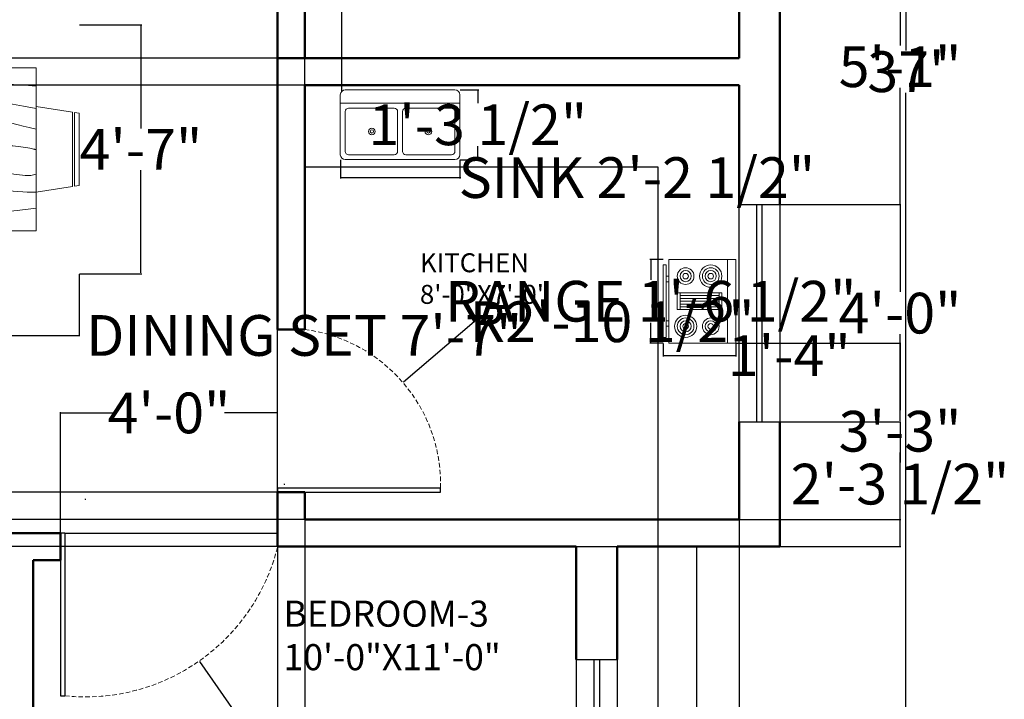
# Model space of a CAD drawing. Units: inches. Extents: x 4033 to 4435, y 499 to 1031.
# Tile 3 of 4: x 4217 to 4435, y 614 to 765. Entities that reach past the tile are written whole.
import ezdxf

# ---------------------------------------------------------------- set-up
doc = ezdxf.new("R2010")
doc.units = ezdxf.units.IN
doc.header["$MEASUREMENT"] = 0
doc.linetypes.add('DASHEDX2', pattern=[1.5, 1, -0.5])
for name, color, linetype, lineweight in [('A-ANNO-DIMS', 2, 'Continuous', 18), ('A-AREA-IDEN', 7, 'Continuous', 18), ('A-DOOR', 3, 'Continuous', 25), ('A-DOOR-SWNG', 3, 'DASHEDX2', 13), ('A-EQPM', 9, 'Continuous', 18), ('A-FLOR-CASE', 8, 'Continuous', 25), ('A-FLOR-FIXT', 8, 'Continuous', 18), ('A-FURN', 8, 'Continuous', 18), ('A-WALL', 7, 'Continuous', 50)]:
    doc.layers.add(name, color=color, linetype=linetype, lineweight=lineweight)
doc.layers.add('A-GLAZ', color=177, linetype='Continuous', lineweight=25, true_color=0x293189)
doc.styles.get("Standard").update_dxf_attribs({"font": 'arial.ttf'})
doc.dimstyles.get("Standard").update_dxf_attribs({"dimtxt": 9, "dimasz": 0.18, "dimexe": 0.18, "dimexo": 0.0625, "dimgap": 0.09, "dimtad": 0, "dimtih": 1, "dimtoh": 1, "dimdec": 0, "dimzin": 0, "dimdsep": 46, "dimlunit": 3, "dimtxsty": 'Standard', "dimcen": 0.09, "dimadec": 0, "dimazin": 0, "dimtfac": 1, "dimtdec": 0, "dimtofl": 0, "dimtmove": 0, "dimatfit": 3, "dimfxl": 1, "dimtolj": 1, "dimtzin": 0, "dimarcsym": 0})

# ---------------------------------------------------------------- blocks, each defined once
blk = doc.blocks.new('Range-Oven - 30 in top')
for p, q in [((0, -3), (30, -3)), ((12, -6), (18, -6)), ((13, -20), (13, -6)), ((14, -6), (14, -20)), ((15, -20), (15, -6)), ((16, -6), (16, -20)), ((17, -20), (17, -6)), ((18, -20), (12, -20)), ((6, -24), (6, -25)), ((8, -25), (8, -24)), ((22, -25), (22, -24)), ((24, -24), (24, -25))]:
    blk.add_line(p, q)
for points in [[(0, -24), (0, 0), (30, 0), (30, -24)], [(12, -21), (12, -5), (18, -5), (18, -21)], [(2, -26), (2, -25), (28, -25), (28, -26)]]:
    blk.add_lwpolyline(points, close=True)
for centre, radius in [((6, -9), 4), ((6, -9), 3), ((6, -9), 2), ((24, -9), 3), ((24, -9), 2), ((6, -9), 1), ((24, -9), 1), ((24, -18), 4), ((6, -18), 3), ((6, -18), 2), ((6, -18), 1), ((24, -18), 3), ((24, -18), 2), ((24, -18), 1)]:
    blk.add_circle(centre, radius)
blk = doc.blocks.new('Sink-double - 36 in top')
for p, q in [((-18, -4), (18, -4)), ((-0.75, -18.5), (-0.75, -6.5)), ((0.75, -6.5), (0.75, -18.5))]:
    blk.add_line(p, q)
for points in [[(-16.5, 0), (16.5, 0)], [(-18, -19.5), (-18, -1.5)], [(18, -1.5), (18, -19.5)], [(-15.5, -5.5), (-1.75, -5.5)], [(1.75, -5.5), (15.5, -5.5)], [(-16.5, -18.5), (-16.5, -6.5)], [(16.5, -6.5), (16.5, -18.5)], [(-1.75, -19.5), (-15.5, -19.5)], [(15.5, -19.5), (1.75, -19.5)], [(16.5, -21), (-16.5, -21)]]:
    blk.add_lwpolyline(points)
for centre, radius in [((-8.5, -12.5), 1), ((8.5, -12.5), 1), ((-8.5, -12.5), 0.5), ((8.5, -12.5), 0.5)]:
    blk.add_circle(centre, radius)
for centre, radius, start, end in [((-16.5, -1.5), 1.5, 90, 180), ((16.5, -1.5), 1.5, 0, 90), ((-15.5, -6.5), 1, 90, 180), ((-1.75, -6.5), 1, 0, 90), ((1.75, -6.5), 1, 90, 180), ((15.5, -6.5), 1, 0, 90), ((-16.5, -19.5), 1.5, 180, 270), ((-15.5, -18.5), 1, 180, 270), ((-1.75, -18.5), 1, 270, 0), ((1.75, -18.5), 1, 180, 270), ((15.5, -18.5), 1, 270, 0), ((16.5, -19.5), 1.5, 270, 0)]:
    blk.add_arc(centre, radius, start, end)
blk = doc.blocks.new('Dining Set - 36 x 72 in.')
for p, q in [((-22, 27.5), (-22.1562, 26.50042)), ((-5.8416, 26.5), (-22.1534, 26.5)), ((-22, 27.5), (-6, 27.5)), ((-5.8437, 26.49966), (-6, 27.5)), ((6, 27.5), (5.8438, 26.50042)), ((22.1584, 26.5), (5.8466, 26.5)), ((6, 27.5), (22, 27.5)), ((22.1563, 26.49966), (22, 27.5)), ((-22.2343, 26.00059), (-23.4847, 17.99762)), ((-22.2304, 26), (-5.7608, 26)), ((-4.5152, 17.99762), (-5.7655, 25.99926)), ((5.7657, 26.00059), (4.5153, 17.99762)), ((5.7696, 26), (22.2392, 26)), ((23.4848, 17.99762), (22.2345, 25.99926)), ((36, 18), (-36, 18)), ((-36, 18), (-36, -18)), ((36, -18), (36, 18)), ((-44.0006, 8.23428), (-35.9976, 9.48474)), ((44.0006, 8.23428), (35.9976, 9.48474)), ((-45.5, 8), (-44.5004, 8.15617)), ((-45.5, 8), (-45.5, -8)), ((-44.5, -8.15843), (-44.5, 8.15338)), ((-44, 8.23041), (-44, -8.23915)), ((44, 8.23041), (44, -8.23915)), ((44.5, -8.15843), (44.5, 8.15338)), ((45.5, 8), (44.5005, 8.15617)), ((45.5, 8), (45.5, -8)), ((-44.4997, -8.15631), (-45.5, -8)), ((-35.9976, -9.48476), (-43.9993, -8.2345)), ((35.9976, -9.48476), (43.9993, -8.2345)), ((44.4997, -8.15631), (45.5, -8)), ((-36, -18), (36, -18)), ((-22.2343, -26.0006), (-23.4847, -17.99762)), ((-4.5152, -17.99762), (-5.7655, -25.99928)), ((5.7657, -26.0006), (4.5153, -17.99762)), ((23.4848, -17.99762), (22.2345, -25.99928)), ((-22.2304, -26), (-5.7608, -26)), ((5.7696, -26), (22.2392, -26)), ((-22, -27.5), (-22.1562, -26.50044)), ((-5.8416, -26.5), (-22.1534, -26.5)), ((-22, -27.5), (-6, -27.5)), ((-5.8437, -26.49967), (-6, -27.5)), ((6, -27.5), (5.8438, -26.50044)), ((22.1584, -26.5), (5.8466, -26.5)), ((6, -27.5), (22, -27.5)), ((22.1563, -26.49967), (22, -27.5))]:
    blk.add_line(p, q)
for points in [[(-36, 15), (-31.1772, 14.97754), (-26.8079, 14.91406), (-22.8538, 14.81543), (-19.276, 14.6875), (-16.0362, 14.53613), (-13.0957, 14.36718), (-10.4159, 14.18652), (-7.9583, 14), (-5.6904, 13.81315), (-3.6035, 13.63021), (-1.6954, 13.45508), (0.0365, 13.29166), (1.5945, 13.14388), (2.9811, 13.01562), (4.1988, 12.9108), (5.25, 12.83333), (6.1393, 12.78613), (6.8802, 12.76823), (7.4883, 12.77767), (7.9792, 12.8125), (8.3685, 12.87077), (8.6719, 12.95052), (8.9049, 13.0498), (9.0833, 13.16666), (9.2205, 13.29899), (9.3216, 13.44401), (9.3895, 13.59879), (9.4271, 13.76041), (9.4373, 13.92594), (9.4232, 14.09245), (9.3875, 14.257), (9.3333, 14.41666), (9.2638, 14.56917), (9.1836, 14.71484), (9.0975, 14.85465), (9.0104, 14.98958), (8.9272, 15.1206), (8.8529, 15.2487), (8.7922, 15.37483), (8.75, 15.5), (8.7305, 15.62467), (8.7344, 15.74739), (8.7617, 15.86621), (8.8125, 15.97916), (8.8867, 16.08431), (8.9844, 16.17968), (9.1055, 16.26334), (9.25, 16.33333), (9.4189, 16.38802), (9.6172, 16.42708), (9.8506, 16.45052), (10.125, 16.45833), (10.4463, 16.45052), (10.8203, 16.42708), (11.2529, 16.38802), (11.75, 16.33333), (12.3184, 16.26318), (12.9694, 16.17838), (13.7151, 16.07991), (14.5677, 15.96875), (15.5395, 15.84586), (16.6426, 15.71224), (17.8893, 15.56884), (19.2917, 15.41666), (20.859, 15.25667), (22.5879, 15.08984), (24.4721, 14.91715), (26.5052, 14.73958), (28.6809, 14.5581), (30.9929, 14.3737), (33.4347, 14.18733), (36, 14)], [(-36, 10), (-28.9766, 10.14274), (-23.1725, 10.20442), (-18.4241, 10.19775), (-14.5677, 10.13541), (-11.4399, 10.03011), (-8.877, 9.89453), (-6.7154, 9.74137), (-4.7917, 9.58333), (-2.9698, 9.43082), (-1.2246, 9.28515), (0.4415, 9.14534), (2.026, 9.01041), (3.5266, 8.87939), (4.9408, 8.7513), (6.266, 8.62516), (7.5, 8.5), (8.6411, 8.37549), (9.6914, 8.2539), (10.6538, 8.13818), (11.5312, 8.03125), (12.3267, 7.93603), (13.043, 7.85547), (13.6831, 7.79248), (14.25, 7.75), (14.7471, 7.7303), (15.1797, 7.73307), (15.5537, 7.75732), (15.875, 7.80208), (16.1494, 7.86637), (16.3828, 7.94922), (16.5811, 8.04964), (16.75, 8.16666), (16.8944, 8.29915), (17.0143, 8.44531), (17.1089, 8.60319), (17.1771, 8.77083), (17.218, 8.94629), (17.2305, 9.1276), (17.2137, 9.31282), (17.1667, 9.5), (17.0895, 9.6875), (16.987, 9.875), (16.8649, 10.0625), (16.7292, 10.25), (16.5856, 10.4375), (16.4401, 10.625), (16.2985, 10.8125), (16.1667, 11), (16.05, 11.18733), (15.9518, 11.3737), (15.8752, 11.5581), (15.8229, 11.73958), (15.798, 11.91715), (15.8034, 12.08984), (15.842, 12.25667), (15.9167, 12.41666), (16.0295, 12.56836), (16.1784, 12.70833), (16.3605, 12.83268), (16.5729, 12.9375), (16.8127, 13.01888), (17.0768, 13.07291), (17.3625, 13.0957), (17.6667, 13.08333), (17.9894, 13.03312), (18.3418, 12.94726), (18.7382, 12.82918), (19.1927, 12.68229), (19.7195, 12.51001), (20.3327, 12.31575), (21.0465, 12.10294), (21.875, 11.875), (22.8357, 11.63354), (23.959, 11.37304), (25.2786, 11.08618), (26.8282, 10.76562), (28.6414, 10.40405), (30.752, 9.99414), (33.1936, 9.52856), (36, 9)], [(-36, 5.5), (-30.7157, 5.3348), (-26.069, 5.20963), (-21.9946, 5.11767), (-18.4271, 5.05208), (-15.3009, 5.00602), (-12.5508, 4.97265), (-10.1112, 4.94515), (-7.9167, 4.91666), (-5.909, 4.88167), (-4.0586, 4.83984), (-2.3429, 4.79215), (-0.7396, 4.73958), (0.7739, 4.6831), (2.22, 4.6237), (3.6213, 4.56233), (5, 4.5), (6.373, 4.43782), (7.7344, 4.3776), (9.0723, 4.32129), (10.375, 4.27083), (11.6309, 4.22819), (12.8281, 4.19531), (13.9551, 4.17415), (15, 4.16666), (15.954, 4.17448), (16.819, 4.19791), (17.6001, 4.23698), (18.3021, 4.29166), (18.9299, 4.36198), (19.4883, 4.44791), (19.9823, 4.54948), (20.4167, 4.66666), (20.7969, 4.79899), (21.1302, 4.94401), (21.4245, 5.09879), (21.6875, 5.26041), (21.9271, 5.42594), (22.1511, 5.59245), (22.3672, 5.757), (22.5834, 5.91666), (22.8065, 6.06868), (23.0404, 6.21093), (23.2879, 6.34147), (23.5521, 6.45833), (23.8358, 6.55957), (24.142, 6.64323), (24.4735, 6.70735), (24.8334, 6.75), (25.2235, 6.76969), (25.642, 6.76692), (26.0858, 6.74267), (26.5521, 6.69791), (27.0379, 6.63362), (27.5404, 6.55078), (28.0565, 6.45036), (28.5834, 6.33333), (29.1242, 6.19987), (29.7071, 6.04687), (30.3661, 5.87044), (31.1354, 5.66666), (32.0493, 5.43164), (33.142, 5.16146), (34.4475, 4.85221), (36, 4.5)], [(-36, -1), (-30.7915, -0.6591), (-26.0195, -0.38216), (-21.6519, -0.16284), (-17.6563, 0.00521), (-14.0005, 0.12833), (-10.6523, 0.21289), (-7.5796, 0.26522), (-4.75, 0.29166), (-2.134, 0.29793), (0.2878, 0.28711), (2.5317, 0.26163), (4.6146, 0.22396), (6.5529, 0.17651), (8.3633, 0.12174), (10.0623, 0.06209), (11.6667, 0), (13.1899, -0.06201), (14.6341, -0.1211), (15.9982, -0.17432), (17.2813, -0.21875), (18.4823, -0.25147), (19.6003, -0.26953), (20.6343, -0.27002), (21.5834, -0.25), (22.4481, -0.20768), (23.2357, -0.14584), (23.9549, -0.06836), (24.6146, 0.02083), (25.2235, 0.11784), (25.7904, 0.21875), (26.3241, 0.31966), (26.8334, 0.41666), (27.3265, 0.50618), (27.8099, 0.58593), (28.2894, 0.65397), (28.7709, 0.70833), (29.2601, 0.74707), (29.763, 0.76823), (30.2855, 0.76985), (30.8334, 0.75), (31.4088, 0.70784), (31.9994, 0.64713), (32.589, 0.57275), (33.1615, 0.48958), (33.7008, 0.4025), (34.1908, 0.3164), (34.6153, 0.23616), (34.9584, 0.16666), (35.2099, 0.11165), (35.3848, 0.07031), (35.504, 0.04069), (35.5886, 0.02083), (35.6594, 0.00879), (35.7377, 0.0026), (35.8442, 0.00032), (36, 0)], [(-36, -6.5), (-27.1843, -6.31267), (-20.084, -6.1263), (-14.469, -5.9419), (-10.1094, -5.76042), (-6.7752, -5.58285), (-4.2363, -5.41016), (-2.2629, -5.24333), (-0.625, -5.08334), (0.8708, -4.93099), (2.2715, -4.78646), (3.5872, -4.64974), (4.8281, -4.52084), (6.0046, -4.39974), (7.127, -4.28646), (8.2053, -4.18099), (9.25, -4.08334), (10.2705, -3.99382), (11.2734, -3.91407), (12.2647, -3.84603), (13.25, -3.79167), (14.2354, -3.75293), (15.2266, -3.73177), (16.2295, -3.73015), (17.25, -3.75), (18.2912, -3.79248), (19.3451, -3.85547), (20.4009, -3.93604), (21.4479, -4.03125), (22.4754, -4.13819), (23.4727, -4.25391), (24.4289, -4.37549), (25.3334, -4.5), (26.1785, -4.62492), (26.9694, -4.74935), (27.7145, -4.87281), (28.4219, -4.99479), (29.1, -5.11483), (29.7572, -5.23242), (30.4016, -5.34709), (31.0417, -5.45834), (31.6837, -5.56437), (32.3262, -5.65821), (32.9658, -5.73153), (33.599, -5.77604), (34.2224, -5.78345), (34.8327, -5.74545), (35.4264, -5.65373), (36, -5.5)], [(-36, -10), (-26.4022, -9.81299), (-18.4675, -9.62891), (-11.9839, -9.45069), (-6.7396, -9.28125), (-2.5226, -9.12354), (0.8789, -8.98047), (3.6769, -8.85498), (6.0833, -8.75), (8.2767, -8.66765), (10.3021, -8.60677), (12.1712, -8.56543), (13.8958, -8.54167), (15.4876, -8.53353), (16.9583, -8.53907), (18.3197, -8.55632), (19.5834, -8.58334), (20.7616, -8.61841), (21.8685, -8.66081), (22.9188, -8.71004), (23.9271, -8.76563), (24.9081, -8.82707), (25.8763, -8.89388), (26.8465, -8.96558), (27.8334, -9.04167), (28.8474, -9.12118), (29.8828, -9.20117), (30.93, -9.27824), (31.9792, -9.34896), (33.0205, -9.40991), (34.0443, -9.45768), (35.0407, -9.48885), (36, -9.5)], [(-36, -14.5), (-30.0881, -14.33513), (-25.0332, -14.21224), (-20.7312, -14.12647), (-17.0781, -14.07292), (-13.97, -14.04671), (-11.3027, -14.04297), (-8.9724, -14.05681), (-6.875, -14.08334), (-4.9224, -14.11833), (-3.0905, -14.16016), (-1.3709, -14.20785), (0.2448, -14.26042), (1.7647, -14.3169), (3.1973, -14.3763), (4.5507, -14.43767), (5.8333, -14.5), (7.0554, -14.5621), (8.235, -14.62175), (9.3922, -14.67652), (10.5469, -14.72396), (11.7192, -14.76164), (12.929, -14.78711), (14.1965, -14.79794), (15.5417, -14.79167), (16.9933, -14.76424), (18.6152, -14.70508), (20.4804, -14.60197), (22.6615, -14.44271), (25.2312, -14.21509), (28.2624, -13.9069), (31.8277, -13.50594), (36, -13)]]:
    blk.add_lwpolyline(points)
blk = doc.blocks.new('*D11')
at = {"layer": 'A-ANNO-DIMS', "color": 0, "lineweight": -2, "transparency": 16777216}
for p, q in [((4305.74, 975.25), (4413.19, 975.25)), ((4413.01, 975.07), (4413.01, 757.94)), ((4413.01, 531.43), (4413.01, 748.56)), ((4349.24, 531.25), (4413.19, 531.25))]:
    blk.add_line(p, q, dxfattribs=at)
at = {"layer": 'A-ANNO-DIMS', "color": 0, "transparency": 16777216}
for points in [[(4412.98, 975.07), (4413.04, 975.07), (4413.01, 975.25)], [(4412.98, 531.43), (4413.04, 531.43), (4413.01, 531.25)]]:
    blk.add_solid(points, dxfattribs=at)
at = {"layer": 'Defpoints', "color": 0, "transparency": 16777216}
for p in [(4305.68, 975.25), (4413.01, 975.25), (4349.18, 531.25)]:
    blk.add_point(p, dxfattribs=at)
at = {"layer": 'A-ANNO-DIMS', "color": 0, "transparency": 16777216, "insert": (4413.01, 753.25), "char_height": 9, "attachment_point": 5}
blk.add_mtext("\\A1;37'", dxfattribs=at)
blk = doc.blocks.new('WIN-60IN')
for p, q in [((0, 0), (0, 9)), ((0, 9), (60, 9)), ((60, 0), (60, 9)), ((0, 5.1), (60, 5.1)), ((0, 3.9), (60, 3.9)), ((0, 0), (60, 0))]:
    blk.add_line(p, q)
blk = doc.blocks.new('DOOR-LEAF-36IN')
for p, q in [((0, 0), (0, 36)), ((1, 36), (0, 36)), ((1, 0), (1, 36)), ((0, 0), (1, 0))]:
    blk.add_line(p, q)
blk = doc.blocks.new('*D24')
at = {"layer": 'A-ANNO-DIMS', "color": 0, "lineweight": -2, "transparency": 16777216}
for p, q in [((4359.35, 711.75), (4356.46, 711.75)), ((4356.64, 711.57), (4356.64, 707.24)), ((4356.64, 693.43), (4356.64, 697.76)), ((4359.35, 693.25), (4356.46, 693.25))]:
    blk.add_line(p, q, dxfattribs=at)
at = {"layer": 'A-ANNO-DIMS', "color": 0, "transparency": 16777216}
for points in [[(4356.61, 711.57), (4356.67, 711.57), (4356.64, 711.75)], [(4356.61, 693.43), (4356.67, 693.43), (4356.64, 693.25)]]:
    blk.add_solid(points, dxfattribs=at)
at = {"layer": 'Defpoints', "color": 0, "transparency": 16777216}
for p in [(4359.41, 711.75), (4356.64, 693.25), (4359.41, 693.25)]:
    blk.add_point(p, dxfattribs=at)
at = {"layer": 'A-ANNO-DIMS', "color": 0, "transparency": 16777216, "insert": (4356.64, 702.5), "char_height": 9, "attachment_point": 5}
blk.add_mtext('\\A1;RANGE 1\'-6 1/2"', dxfattribs=at)
blk = doc.blocks.new('*D25')
at = {"layer": 'A-ANNO-DIMS', "color": 0, "lineweight": -2, "transparency": 16777216}
for p, q in [((4359.41, 693.19), (4359.41, 690.3)), ((4375.44, 693.19), (4375.44, 690.3)), ((4359.59, 690.48), (4375.26, 690.48)), ((4375.44, 690.48), (4375.62, 690.48))]:
    blk.add_line(p, q, dxfattribs=at)
at = {"layer": 'A-ANNO-DIMS', "color": 0, "transparency": 16777216}
for points in [[(4359.59, 690.51), (4359.59, 690.45), (4359.41, 690.48)], [(4375.26, 690.51), (4375.26, 690.45), (4375.44, 690.48)]]:
    blk.add_solid(points, dxfattribs=at)
at = {"layer": 'Defpoints', "color": 0, "transparency": 16777216}
for p in [(4359.41, 693.25), (4375.44, 693.25), (4375.44, 690.48)]:
    blk.add_point(p, dxfattribs=at)
at = {"layer": 'A-ANNO-DIMS', "color": 0, "transparency": 16777216, "insert": (4387.25, 690.48), "char_height": 9, "attachment_point": 5}
blk.add_mtext('\\A1;1\'-4"', dxfattribs=at)
blk = doc.blocks.new('*D26')
at = {"layer": 'A-ANNO-DIMS', "color": 0, "lineweight": -2, "transparency": 16777216}
for p, q in [((4288.04, 733.74), (4288.04, 729.66)), ((4314.47, 733.74), (4314.47, 729.66)), ((4288.22, 729.84), (4314.29, 729.84)), ((4314.47, 729.84), (4314.65, 729.84))]:
    blk.add_line(p, q, dxfattribs=at)
at = {"layer": 'A-ANNO-DIMS', "color": 0, "transparency": 16777216}
for points in [[(4288.22, 729.87), (4288.22, 729.81), (4288.04, 729.84)], [(4314.29, 729.87), (4314.29, 729.81), (4314.47, 729.84)]]:
    blk.add_solid(points, dxfattribs=at)
at = {"layer": 'Defpoints', "color": 0, "transparency": 16777216}
for p in [(4288.04, 733.8), (4314.47, 733.8), (4314.47, 729.84)]:
    blk.add_point(p, dxfattribs=at)
at = {"layer": 'A-ANNO-DIMS', "color": 0, "transparency": 16777216, "insert": (4353.58, 729.84), "char_height": 9, "attachment_point": 5}
blk.add_mtext('\\A1;SINK 2\'-2 1/2"', dxfattribs=at)
blk = doc.blocks.new('*D27')
at = {"layer": 'A-ANNO-DIMS', "color": 0, "lineweight": -2, "transparency": 16777216}
for p, q in [((4314.53, 749.22), (4318.61, 749.22)), ((4318.43, 749.04), (4318.43, 746.26)), ((4318.43, 733.98), (4318.43, 736.76)), ((4314.53, 733.8), (4318.61, 733.8))]:
    blk.add_line(p, q, dxfattribs=at)
at = {"layer": 'A-ANNO-DIMS', "color": 0, "transparency": 16777216}
for points in [[(4318.4, 749.04), (4318.46, 749.04), (4318.43, 749.22)], [(4318.4, 733.98), (4318.46, 733.98), (4318.43, 733.8)]]:
    blk.add_solid(points, dxfattribs=at)
at = {"layer": 'Defpoints', "color": 0, "transparency": 16777216}
for p in [(4314.47, 749.22), (4318.43, 749.22), (4314.47, 733.8)]:
    blk.add_point(p, dxfattribs=at)
at = {"layer": 'A-ANNO-DIMS', "color": 0, "transparency": 16777216, "insert": (4318.43, 741.51), "char_height": 9, "attachment_point": 5}
blk.add_mtext('\\A1;1\'-3 1/2"', dxfattribs=at)
blk = doc.blocks.new('*D30')
at = {"layer": 'A-ANNO-DIMS', "color": 0, "lineweight": -2, "transparency": 16777216}
for p, q in [((4139.32, 708.52), (4139.32, 694.75)), ((4230.32, 708.52), (4230.32, 694.75)), ((4139.5, 694.93), (4230.14, 694.93)), ((4230.32, 694.93), (4230.5, 694.93))]:
    blk.add_line(p, q, dxfattribs=at)
at = {"layer": 'A-ANNO-DIMS', "color": 0, "transparency": 16777216}
for points in [[(4139.5, 694.96), (4139.5, 694.9), (4139.32, 694.93)], [(4230.14, 694.96), (4230.14, 694.9), (4230.32, 694.93)]]:
    blk.add_solid(points, dxfattribs=at)
at = {"layer": 'Defpoints', "color": 0, "transparency": 16777216}
for p in [(4139.32, 708.58), (4230.32, 708.58), (4230.32, 694.93)]:
    blk.add_point(p, dxfattribs=at)
at = {"layer": 'A-ANNO-DIMS', "color": 0, "transparency": 16777216, "insert": (4280.05, 694.93), "char_height": 9, "attachment_point": 5}
blk.add_mtext('\\A1;DINING SET 7\'-7"', dxfattribs=at)
blk = doc.blocks.new('*D31')
at = {"layer": 'A-ANNO-DIMS', "color": 0, "lineweight": -2, "transparency": 16777216}
for p, q in [((4230.39, 763.58), (4244.15, 763.58)), ((4243.97, 763.4), (4243.97, 740.67)), ((4243.97, 708.76), (4243.97, 731.49)), ((4230.39, 708.58), (4244.15, 708.58))]:
    blk.add_line(p, q, dxfattribs=at)
at = {"layer": 'A-ANNO-DIMS', "color": 0, "transparency": 16777216}
for points in [[(4243.94, 763.4), (4244, 763.4), (4243.97, 763.58)], [(4243.94, 708.76), (4244, 708.76), (4243.97, 708.58)]]:
    blk.add_solid(points, dxfattribs=at)
at = {"layer": 'Defpoints', "color": 0, "transparency": 16777216}
for p in [(4230.32, 763.58), (4243.97, 763.58), (4230.32, 708.58)]:
    blk.add_point(p, dxfattribs=at)
at = {"layer": 'A-ANNO-DIMS', "color": 0, "transparency": 16777216, "insert": (4243.97, 736.08), "char_height": 9, "attachment_point": 5}
blk.add_mtext('\\A1;4\'-7"', dxfattribs=at)
blk = doc.blocks.new('*D37')
at = {"layer": 'A-ANNO-DIMS', "color": 0, "lineweight": -2, "transparency": 16777216}
for p, q in [((4340.24, 648.25), (4366.91, 648.25)), ((4366.73, 648.07), (4366.73, 598.94)), ((4366.73, 540.43), (4366.73, 589.56)), ((4340.24, 540.25), (4366.91, 540.25))]:
    blk.add_line(p, q, dxfattribs=at)
at = {"layer": 'A-ANNO-DIMS', "color": 0, "transparency": 16777216}
for points in [[(4366.7, 648.07), (4366.76, 648.07), (4366.73, 648.25)], [(4366.7, 540.43), (4366.76, 540.43), (4366.73, 540.25)]]:
    blk.add_solid(points, dxfattribs=at)
at = {"layer": 'Defpoints', "color": 0, "transparency": 16777216}
for p in [(4340.18, 648.25), (4340.18, 540.25), (4366.73, 540.25)]:
    blk.add_point(p, dxfattribs=at)
at = {"layer": 'A-ANNO-DIMS', "color": 0, "transparency": 16777216, "insert": (4366.73, 594.25), "char_height": 9, "attachment_point": 5}
blk.add_mtext('\\A1;9\'-0"', dxfattribs=at)
blk = doc.blocks.new('*D45')
at = {"layer": 'A-ANNO-DIMS', "color": 0, "lineweight": -2, "transparency": 16777216}
for p, q in [((4226.18, 651.31), (4226.18, 677.98)), ((4226.36, 677.8), (4237.94, 677.8)), ((4274, 677.8), (4262.41, 677.8)), ((4274.18, 651.31), (4274.18, 677.98))]:
    blk.add_line(p, q, dxfattribs=at)
at = {"layer": 'A-ANNO-DIMS', "color": 0, "transparency": 16777216}
for points in [[(4226.36, 677.83), (4226.36, 677.77), (4226.18, 677.8)], [(4274, 677.83), (4274, 677.77), (4274.18, 677.8)]]:
    blk.add_solid(points, dxfattribs=at)
at = {"layer": 'Defpoints', "color": 0, "transparency": 16777216}
for p in [(4274.18, 677.8), (4226.18, 651.25), (4274.18, 651.25)]:
    blk.add_point(p, dxfattribs=at)
at = {"layer": 'A-ANNO-DIMS', "color": 0, "transparency": 16777216, "insert": (4250.18, 677.8), "char_height": 9, "attachment_point": 5}
blk.add_mtext('\\A1;4\'-0"', dxfattribs=at)
blk = doc.blocks.new('*D50')
at = {"layer": 'A-ANNO-DIMS', "color": 0, "lineweight": -2, "transparency": 16777216}
for p, q in [((4385.24, 723.87), (4411.91, 723.87)), ((4411.73, 723.69), (4411.73, 704.56)), ((4411.73, 676.05), (4411.73, 695.19)), ((4385.24, 675.87), (4411.91, 675.87))]:
    blk.add_line(p, q, dxfattribs=at)
at = {"layer": 'A-ANNO-DIMS', "color": 0, "transparency": 16777216}
for points in [[(4411.7, 723.69), (4411.76, 723.69), (4411.73, 723.87)], [(4411.7, 676.05), (4411.76, 676.05), (4411.73, 675.87)]]:
    blk.add_solid(points, dxfattribs=at)
at = {"layer": 'Defpoints', "color": 0, "transparency": 16777216}
for p in [(4385.18, 723.87), (4411.73, 723.87), (4385.18, 675.87)]:
    blk.add_point(p, dxfattribs=at)
at = {"layer": 'A-ANNO-DIMS', "color": 0, "transparency": 16777216, "insert": (4411.73, 699.87), "char_height": 9, "attachment_point": 5}
blk.add_mtext('\\A1;4\'-0"', dxfattribs=at)
blk = doc.blocks.new('*D52')
at = {"layer": 'A-ANNO-DIMS', "color": 0, "lineweight": -2, "transparency": 16777216}
for p, q in [((4385.24, 675.87), (4411.91, 675.87)), ((4411.73, 675.69), (4411.73, 666.81)), ((4411.73, 648.43), (4411.73, 657.32)), ((4385.24, 648.25), (4411.91, 648.25))]:
    blk.add_line(p, q, dxfattribs=at)
at = {"layer": 'A-ANNO-DIMS', "color": 0, "transparency": 16777216}
for points in [[(4411.7, 675.69), (4411.76, 675.69), (4411.73, 675.87)], [(4411.7, 648.43), (4411.76, 648.43), (4411.73, 648.25)]]:
    blk.add_solid(points, dxfattribs=at)
at = {"layer": 'Defpoints', "color": 0, "transparency": 16777216}
for p in [(4385.18, 675.87), (4411.73, 675.87), (4385.18, 648.25)]:
    blk.add_point(p, dxfattribs=at)
at = {"layer": 'A-ANNO-DIMS', "color": 0, "transparency": 16777216, "insert": (4411.73, 662.06), "char_height": 9, "attachment_point": 5}
blk.add_mtext('\\A1;2\'-3 1/2"', dxfattribs=at)
blk = doc.blocks.new('*D53')
at = {"layer": 'A-ANNO-DIMS', "color": 0, "lineweight": -2, "transparency": 16777216}
for p, q in [((4385.24, 784.85), (4411.91, 784.85)), ((4411.73, 784.67), (4411.73, 759.05)), ((4411.73, 724.05), (4411.73, 749.68)), ((4385.24, 723.87), (4411.91, 723.87))]:
    blk.add_line(p, q, dxfattribs=at)
at = {"layer": 'A-ANNO-DIMS', "color": 0, "transparency": 16777216}
for points in [[(4411.7, 784.67), (4411.76, 784.67), (4411.73, 784.85)], [(4411.7, 724.05), (4411.76, 724.05), (4411.73, 723.87)]]:
    blk.add_solid(points, dxfattribs=at)
at = {"layer": 'Defpoints', "color": 0, "transparency": 16777216}
for p in [(4385.18, 784.85), (4411.73, 784.85), (4385.18, 723.87)]:
    blk.add_point(p, dxfattribs=at)
at = {"layer": 'A-ANNO-DIMS', "color": 0, "transparency": 16777216, "insert": (4411.73, 754.36), "char_height": 9, "attachment_point": 5}
blk.add_mtext('\\A1;5\'-1"', dxfattribs=at)
blk = doc.blocks.new('*D54')
at = {"layer": 'A-ANNO-DIMS', "color": 0, "lineweight": -2, "transparency": 16777216}
for p, q in [((4280.12, 750.25), (4058.45, 750.25)), ((4058.63, 750.07), (4058.63, 706.94)), ((4058.63, 654.43), (4058.63, 697.56)), ((4280.12, 654.25), (4058.45, 654.25))]:
    blk.add_line(p, q, dxfattribs=at)
at = {"layer": 'A-ANNO-DIMS', "color": 0, "transparency": 16777216}
for points in [[(4058.6, 750.07), (4058.66, 750.07), (4058.63, 750.25)], [(4058.6, 654.43), (4058.66, 654.43), (4058.63, 654.25)]]:
    blk.add_solid(points, dxfattribs=at)
at = {"layer": 'Defpoints', "color": 0, "transparency": 16777216}
for p in [(4058.63, 750.25), (4280.18, 750.25), (4280.18, 654.25)]:
    blk.add_point(p, dxfattribs=at)
at = {"layer": 'A-ANNO-DIMS', "color": 0, "transparency": 16777216, "insert": (4058.63, 702.25), "char_height": 9, "attachment_point": 5}
blk.add_mtext('\\A1;8\'-0"', dxfattribs=at)
blk = doc.blocks.new('*D55')
at = {"layer": 'A-ANNO-DIMS', "color": 0, "lineweight": -2, "transparency": 16777216}
for p, q in [((4280.12, 756.25), (4058.45, 756.25)), ((4058.63, 756.25), (4058.63, 756.43)), ((4058.63, 756.43), (4058.81, 756.43)), ((4058.63, 750.43), (4058.63, 756.07)), ((4280.12, 750.25), (4058.45, 750.25))]:
    blk.add_line(p, q, dxfattribs=at)
at = {"layer": 'A-ANNO-DIMS', "color": 0, "transparency": 16777216}
for points in [[(4058.6, 756.07), (4058.66, 756.07), (4058.63, 756.25)], [(4058.6, 750.43), (4058.66, 750.43), (4058.63, 750.25)]]:
    blk.add_solid(points, dxfattribs=at)
at = {"layer": 'Defpoints', "color": 0, "transparency": 16777216}
for p in [(4058.63, 756.25), (4280.18, 756.25), (4280.18, 750.25)]:
    blk.add_point(p, dxfattribs=at)
at = {"layer": 'A-ANNO-DIMS', "color": 0, "transparency": 16777216, "insert": (4070.86, 756.43), "char_height": 9, "attachment_point": 5}
blk.add_mtext('\\A1;0\'-6"', dxfattribs=at)
blk = doc.blocks.new('*D56')
at = {"layer": 'A-ANNO-DIMS', "color": 0, "lineweight": -2, "transparency": 16777216}
for p, q in [((4280.18, 654.19), (4280.18, 504.52)), ((4274.18, 648.19), (4274.18, 504.52)), ((4274.18, 504.7), (4274, 504.7)), ((4280, 504.7), (4274.36, 504.7))]:
    blk.add_line(p, q, dxfattribs=at)
at = {"layer": 'A-ANNO-DIMS', "color": 0, "transparency": 16777216}
for points in [[(4274.36, 504.73), (4274.36, 504.67), (4274.18, 504.7)], [(4280, 504.73), (4280, 504.67), (4280.18, 504.7)]]:
    blk.add_solid(points, dxfattribs=at)
at = {"layer": 'Defpoints', "color": 0, "transparency": 16777216}
for p in [(4280.18, 654.25), (4274.18, 648.25), (4274.18, 504.7)]:
    blk.add_point(p, dxfattribs=at)
at = {"layer": 'A-ANNO-DIMS', "color": 0, "transparency": 16777216, "insert": (4261.95, 504.7), "char_height": 9, "attachment_point": 5}
blk.add_mtext('\\A1;0\'-6"', dxfattribs=at)
blk = doc.blocks.new('*D58')
at = {"layer": 'A-ANNO-DIMS', "color": 0, "lineweight": -2, "transparency": 16777216}
for p, q in [((4274.12, 660.25), (4058.45, 660.25)), ((4058.63, 660.07), (4058.63, 658.94)), ((4058.63, 648.43), (4058.63, 649.56)), ((4274.12, 648.25), (4058.45, 648.25))]:
    blk.add_line(p, q, dxfattribs=at)
at = {"layer": 'A-ANNO-DIMS', "color": 0, "transparency": 16777216}
for points in [[(4058.6, 660.07), (4058.66, 660.07), (4058.63, 660.25)], [(4058.6, 648.43), (4058.66, 648.43), (4058.63, 648.25)]]:
    blk.add_solid(points, dxfattribs=at)
at = {"layer": 'Defpoints', "color": 0, "transparency": 16777216}
for p in [(4058.63, 660.25), (4274.18, 660.25), (4274.18, 648.25)]:
    blk.add_point(p, dxfattribs=at)
at = {"layer": 'A-ANNO-DIMS', "color": 0, "transparency": 16777216, "insert": (4058.63, 654.25), "char_height": 9, "attachment_point": 5}
blk.add_mtext('\\A1;1\'-0"', dxfattribs=at)
blk = doc.blocks.new('*D59')
at = {"layer": 'A-ANNO-DIMS', "color": 0, "lineweight": -2, "transparency": 16777216}
for p, q in [((4358.18, 654.19), (4358.18, 504.52)), ((4376.18, 654.19), (4376.18, 504.52)), ((4358.36, 504.7), (4376, 504.7)), ((4376.18, 504.7), (4376.36, 504.7))]:
    blk.add_line(p, q, dxfattribs=at)
at = {"layer": 'A-ANNO-DIMS', "color": 0, "transparency": 16777216}
for points in [[(4358.36, 504.73), (4358.36, 504.67), (4358.18, 504.7)], [(4376, 504.73), (4376, 504.67), (4376.18, 504.7)]]:
    blk.add_solid(points, dxfattribs=at)
at = {"layer": 'Defpoints', "color": 0, "transparency": 16777216}
for p in [(4358.18, 654.25), (4376.18, 654.25), (4376.18, 504.7)]:
    blk.add_point(p, dxfattribs=at)
at = {"layer": 'A-ANNO-DIMS', "color": 0, "transparency": 16777216, "insert": (4387.99, 504.7), "char_height": 9, "attachment_point": 5}
blk.add_mtext('\\A1;1\'-6"', dxfattribs=at)
blk = doc.blocks.new('*D60')
at = {"layer": 'A-ANNO-DIMS', "color": 0, "lineweight": -2, "transparency": 16777216}
for p, q in [((4280.18, 750.31), (4280.18, 1001.98)), ((4280.36, 1001.8), (4288.18, 1001.8)), ((4288.36, 748.96), (4288.36, 1001.98)), ((4288.36, 1001.8), (4288.54, 1001.8))]:
    blk.add_line(p, q, dxfattribs=at)
at = {"layer": 'A-ANNO-DIMS', "color": 0, "transparency": 16777216}
for points in [[(4280.36, 1001.83), (4280.36, 1001.77), (4280.18, 1001.8)], [(4288.18, 1001.83), (4288.18, 1001.77), (4288.36, 1001.8)]]:
    blk.add_solid(points, dxfattribs=at)
at = {"layer": 'Defpoints', "color": 0, "transparency": 16777216}
for p in [(4288.36, 1001.8), (4280.18, 750.25), (4288.36, 748.89)]:
    blk.add_point(p, dxfattribs=at)
at = {"layer": 'A-ANNO-DIMS', "color": 0, "transparency": 16777216, "insert": (4300.59, 1001.8), "char_height": 9, "attachment_point": 5}
blk.add_mtext('\\A1;0\'-8"', dxfattribs=at)
blk = doc.blocks.new('*D61')
at = {"layer": 'A-ANNO-DIMS', "color": 0, "lineweight": -2, "transparency": 16777216}
for p, q in [((4375.5, 693.25), (4411.91, 693.25)), ((4411.73, 693.07), (4411.73, 678.44)), ((4411.73, 654.43), (4411.73, 669.06)), ((4376.24, 654.25), (4411.91, 654.25))]:
    blk.add_line(p, q, dxfattribs=at)
at = {"layer": 'A-ANNO-DIMS', "color": 0, "transparency": 16777216}
for points in [[(4411.7, 693.07), (4411.76, 693.07), (4411.73, 693.25)], [(4411.7, 654.43), (4411.76, 654.43), (4411.73, 654.25)]]:
    blk.add_solid(points, dxfattribs=at)
at = {"layer": 'Defpoints', "color": 0, "transparency": 16777216}
for p in [(4375.44, 693.25), (4411.73, 693.25), (4376.18, 654.25)]:
    blk.add_point(p, dxfattribs=at)
at = {"layer": 'A-ANNO-DIMS', "color": 0, "transparency": 16777216, "insert": (4411.73, 673.75), "char_height": 9, "attachment_point": 5}
blk.add_mtext('\\A1;3\'-3"', dxfattribs=at)
blk = doc.blocks.new('*D62')
at = {"layer": 'A-ANNO-DIMS', "color": 0, "lineweight": -2, "transparency": 16777216}
for p, q in [((4231.63, 658.74), (4231.81, 658.74)), ((4231.72, 658.65), (4231.72, 658.83)), ((4271.93, 601.48), (4256.96, 622.81)), ((4272.11, 601.48), (4271.93, 601.48))]:
    blk.add_line(p, q, dxfattribs=at)
at = {"layer": 'A-ANNO-DIMS', "color": 0, "transparency": 16777216}
blk.add_solid([(4256.98, 622.82), (4256.93, 622.79), (4256.85, 622.95)], dxfattribs=at)
at = {"layer": 'Defpoints', "color": 0, "transparency": 16777216}
for p in [(4231.72, 658.74), (4256.85, 622.95)]:
    blk.add_point(p, dxfattribs=at)
at = {"layer": 'A-ANNO-DIMS', "color": 0, "transparency": 16777216, "insert": (4298.96, 601.48), "char_height": 9, "attachment_point": 5}
blk.add_mtext('\\A1;R3\'-7 1/2"', dxfattribs=at)
blk = doc.blocks.new('*D65')
at = {"layer": 'A-ANNO-DIMS', "color": 0, "lineweight": -2, "transparency": 16777216}
for p, q in [((4317.59, 697.96), (4302.02, 684.62)), ((4317.77, 697.96), (4317.59, 697.96)), ((4275.62, 662.06), (4275.8, 662.06)), ((4275.71, 661.97), (4275.71, 662.15))]:
    blk.add_line(p, q, dxfattribs=at)
at = {"layer": 'A-ANNO-DIMS', "color": 0, "transparency": 16777216}
blk.add_solid([(4302, 684.64), (4302.04, 684.6), (4301.89, 684.5)], dxfattribs=at)
at = {"layer": 'Defpoints', "color": 0, "transparency": 16777216}
for p in [(4301.89, 684.5), (4275.71, 662.06)]:
    blk.add_point(p, dxfattribs=at)
at = {"layer": 'A-ANNO-DIMS', "color": 0, "transparency": 16777216, "insert": (4348.11, 697.96), "char_height": 9, "attachment_point": 5}
blk.add_mtext('\\A1;R2\'-10 1/2"', dxfattribs=at)

msp = doc.modelspace()

# ---------------------------------------------------------------- linework, layer by layer
at = {"layer": 'A-DOOR'}
for p, q in [((4274.18, 660.75), (4274.18, 696.25)), ((4227.18, 651.25), (4274.18, 651.25))]:
    msp.add_line(p, q, dxfattribs=at)
at = {"layer": 'A-DOOR-SWNG'}
for centre, radius, start, end in [((4275.71, 662.06), 34.48, 358.648, 82.5546), ((4231.72, 658.74), 43.73, 264.0322, 346.1153)]:
    msp.add_arc(centre, radius, start, end, dxfattribs=at)
at = {"layer": 'A-FLOR-CASE'}
for p, q in [((4280.18, 732.25), (4358.18, 732.25)), ((4358.18, 732.25), (4358.18, 654.25))]:
    msp.add_line(p, q, dxfattribs=at)
at = {"layer": 'A-GLAZ'}
for p, q in [((4376.18, 723.87), (4385.18, 723.87)), ((4376.18, 675.87), (4376.18, 723.87)), ((4380.08, 675.87), (4380.08, 723.87)), ((4381.28, 675.87), (4381.28, 723.87)), ((4385.18, 723.87), (4385.18, 675.87)), ((4376.18, 675.87), (4385.18, 675.87))]:
    msp.add_line(p, q, dxfattribs=at)
at = {"layer": 'A-WALL'}
for p, q in [((4274.18, 785.46), (4274.18, 756.25)), ((4280.18, 785.46), (4280.18, 756.25)), ((4376.18, 784.85), (4376.18, 756.25)), ((4385.18, 784.85), (4385.18, 723.87)), ((4274.18, 756.25), (4376.18, 756.25)), ((4274.18, 756.25), (4274.18, 696.25)), ((4280.18, 750.25), (4376.18, 750.25)), ((4280.18, 750.25), (4280.18, 696.25)), ((4376.18, 750.25), (4376.18, 723.87)), ((4274.18, 696.25), (4280.18, 696.25)), ((4376.18, 675.87), (4376.18, 654.25)), ((4385.18, 675.87), (4385.18, 648.25)), ((4274.18, 660.25), (4280.18, 660.25)), ((4274.18, 660.25), (4274.18, 648.25)), ((4280.18, 660.25), (4280.18, 654.25)), ((4280.18, 654.25), (4376.18, 654.25)), ((4226.18, 651.25), (4214.18, 651.25)), ((4226.18, 645.25), (4226.18, 651.25)), ((4274.18, 648.25), (4340.18, 648.25)), ((4340.18, 623.3), (4340.18, 648.25)), ((4349.18, 648.25), (4385.18, 648.25)), ((4349.18, 623.3), (4349.18, 648.25)), ((4220.18, 540.25), (4220.18, 645.25)), ((4226.18, 645.25), (4220.18, 645.25))]:
    msp.add_line(p, q, dxfattribs=at)

# ---------------------------------------------------------------- block references
at = {"layer": 'A-DOOR'}
for p, rotation in [((4274.18, 661.25), 270.0000000000003), ((4227.18, 651.25), 180)]:
    msp.add_blockref('DOOR-LEAF-36IN', p, dxfattribs=dict(at, rotation=rotation))
at = {"layer": 'A-EQPM', "xscale": 0.6165999963959906, "yscale": 0.6165999963959906, "zscale": 0.6165999963959906, "rotation": 270.0000000000005}
msp.add_blockref('Range-Oven - 30 in top', (4375.44, 711.75), dxfattribs=at)
at = {"layer": 'A-FLOR-FIXT', "xscale": 0.7341058115954854, "yscale": 0.7341058115954854, "zscale": 0.7341058115954854}
msp.add_blockref('Sink-double - 36 in top', (4301.25, 749.22), dxfattribs=at)
at = {"layer": 'A-FURN'}
msp.add_blockref('Dining Set - 36 x 72 in.', (4184.82, 736.08), dxfattribs=at)
at = {"layer": 'A-GLAZ', "rotation": 270.0000000000002}
msp.add_blockref('WIN-60IN', (4340.18, 623.3), dxfattribs=at)

# ---------------------------------------------------------------- texts
at = {"layer": 'A-AREA-IDEN', "attachment_point": 1}
for s, width, gutter_width, insert, char_height in [('KITCHEN\\P8\'-0"X7\'-0"', 1.5551, 20.96, (4305.62, 713.1), 4.1916), ('BEDROOM-3\\P10\'-0"X11\'-0"', 2.1401, 28.84, (4275.48, 636.3), 5.7683)]:
    msp.add_mtext_dynamic_manual_height_columns(s, width=width, gutter_width=gutter_width, heights=[0], dxfattribs=dict(at, insert=insert, char_height=char_height))

# ---------------------------------------------------------------- dimensions: what is measured, and where the dimension line sits
at = {"layer": 'A-ANNO-DIMS'}
for base, p1, p2, picture, middle in [((4288.36, 1001.8), (4280.18, 750.25), (4288.36, 748.89), '*D60', (4300.59, 1001.8)), ((4274.18, 677.8), (4226.18, 651.25), (4274.18, 651.25), '*D45', (4250.18, 677.8)), ((4274.18, 504.7), (4280.18, 654.25), (4274.18, 648.25), '*D56', (4261.95, 504.7)), ((4376.18, 504.7), (4358.18, 654.25), (4376.18, 654.25), '*D59', (4387.99, 504.7))]:
    dim = msp.add_linear_dim(base=base, p1=p1, p2=p2, dimstyle='Standard', override={"dimdec": 1, "dimlfac": 1, "dimrnd": 0, "dimzin": 1, "dimdsep": 46, "dimlunit": 4, "dimfrac": 2}, dxfattribs=at)
    dim.commit()
    dim.dimension.update_dxf_attribs({"geometry": picture, "text_midpoint": middle})
for base, p1, p2, angle, override, picture, middle in [((4413.01, 975.25), (4349.18, 531.25), (4305.68, 975.25), 90, {"dimclrd": 0, "dimclre": 0, "dimclrt": 0}, '*D11', (4413.01, 753.25)), ((4411.73, 784.85), (4385.18, 723.87), (4385.18, 784.85), 90, {"dimdec": 1, "dimlfac": 1, "dimrnd": 0, "dimzin": 1, "dimdsep": 46, "dimlunit": 4, "dimfrac": 2}, '*D53', (4411.73, 754.36)), ((4058.63, 756.25), (4280.18, 750.25), (4280.18, 756.25), 90, {"dimdec": 1, "dimlfac": 1, "dimrnd": 0, "dimzin": 1, "dimdsep": 46, "dimlunit": 4, "dimfrac": 2}, '*D55', (4070.86, 756.43)), ((4243.97, 763.58), (4230.32, 708.58), (4230.32, 763.58), 90, {"dimdec": 1, "dimlfac": 1, "dimrnd": 0, "dimzin": 1, "dimdsep": 46, "dimlunit": 4, "dimfrac": 2}, '*D31', (4243.97, 736.08)), ((4318.43, 749.22), (4314.47, 733.8), (4314.47, 749.22), 90, {"dimdec": 1, "dimlfac": 1, "dimrnd": 0, "dimzin": 1, "dimdsep": 46, "dimlunit": 4, "dimfrac": 2}, '*D27', (4318.43, 741.51)), ((4058.63, 750.25), (4280.18, 654.25), (4280.18, 750.25), 90, {"dimdec": 1, "dimlfac": 1, "dimrnd": 0, "dimzin": 1, "dimdsep": 46, "dimlunit": 4, "dimfrac": 2}, '*D54', (4058.63, 702.25)), ((4411.73, 723.87), (4385.18, 675.87), (4385.18, 723.87), 90, {"dimdec": 1, "dimlfac": 1, "dimrnd": 0, "dimzin": 1, "dimdsep": 46, "dimlunit": 4, "dimfrac": 2}, '*D50', (4411.73, 699.87)), ((4375.44, 690.48), (4359.41, 693.25), (4375.44, 693.25), 0, {"dimdec": 1, "dimlfac": 1, "dimrnd": 0, "dimzin": 1, "dimdsep": 46, "dimlunit": 4, "dimfrac": 2}, '*D25', (4387.25, 690.48)), ((4411.73, 693.25), (4376.18, 654.25), (4375.44, 693.25), 90, {"dimdec": 1, "dimlfac": 1, "dimrnd": 0, "dimzin": 1, "dimdsep": 46, "dimlunit": 4, "dimfrac": 2}, '*D61', (4411.73, 673.75)), ((4411.73, 675.87), (4385.18, 648.25), (4385.18, 675.87), 90, {"dimdec": 1, "dimlfac": 1, "dimrnd": 0, "dimzin": 1, "dimdsep": 46, "dimlunit": 4, "dimfrac": 2}, '*D52', (4411.73, 662.06)), ((4058.63, 660.25), (4274.18, 648.25), (4274.18, 660.25), 90, {"dimdec": 1, "dimlfac": 1, "dimrnd": 0, "dimzin": 1, "dimdsep": 46, "dimlunit": 4, "dimfrac": 2}, '*D58', (4058.63, 654.25)), ((4366.73, 540.25), (4340.18, 648.25), (4340.18, 540.25), 270, {"dimdec": 1, "dimlfac": 1, "dimrnd": 0, "dimzin": 1, "dimdsep": 46, "dimlunit": 4, "dimfrac": 2}, '*D37', (4366.73, 594.25))]:
    dim = msp.add_linear_dim(base=base, p1=p1, p2=p2, angle=angle, dimstyle='Standard', override=override, dxfattribs=at)
    dim.commit()
    dim.dimension.update_dxf_attribs({"geometry": picture, "text_midpoint": middle})
for base, p1, p2, text, picture, middle in [((4314.47, 729.84), (4288.04, 733.8), (4314.47, 733.8), 'SINK <>', '*D26', (4353.58, 729.84)), ((4230.32, 694.93), (4139.32, 708.58), (4230.32, 708.58), 'DINING SET <>', '*D30', (4280.05, 694.93))]:
    dim = msp.add_linear_dim(base=base, p1=p1, p2=p2, text=text, dimstyle='Standard', override={"dimdec": 1, "dimlfac": 1, "dimrnd": 0, "dimzin": 1, "dimdsep": 46, "dimlunit": 4, "dimfrac": 2}, dxfattribs=at)
    dim.commit()
    dim.dimension.update_dxf_attribs({"geometry": picture, "text_midpoint": middle})
dim = msp.add_linear_dim(base=(4356.64, 693.25), p1=(4359.41, 711.75), p2=(4359.41, 693.25), angle=270, text='RANGE <>', dimstyle='Standard', override={"dimdec": 1, "dimlfac": 1, "dimrnd": 0, "dimzin": 1, "dimdsep": 46, "dimlunit": 4, "dimfrac": 2}, dxfattribs=at)
dim.commit()
dim.dimension.update_dxf_attribs({"geometry": '*D24', "text_midpoint": (4356.64, 702.5)})
for center, mpoint, picture, middle in [((4275.71, 662.06), (4301.89, 684.5), '*D65', (4348.11, 697.96)), ((4231.72, 658.74), (4256.85, 622.95), '*D62', (4298.96, 601.48))]:
    dim = msp.add_radius_dim(center=center, mpoint=mpoint, dimstyle='Standard', override={"dimdec": 1, "dimlfac": 1, "dimrnd": 0, "dimzin": 1, "dimdsep": 46, "dimlunit": 4, "dimfrac": 2}, dxfattribs=at)
    dim.commit()
    dim.dimension.update_dxf_attribs({"geometry": picture, "text_midpoint": middle, "dimtype": 164})

doc.saveas('drawing.dxf')
